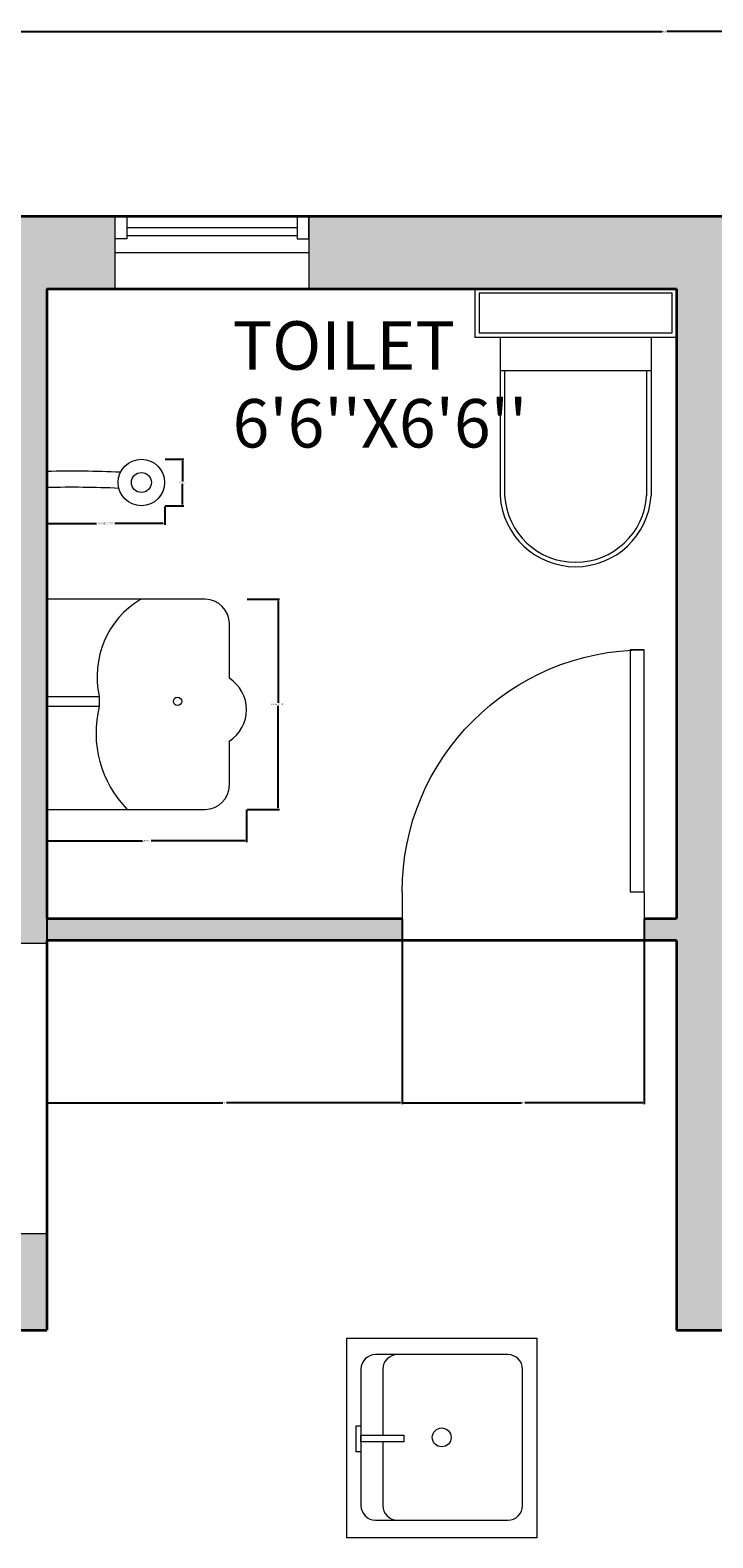
# Model space of a CAD drawing. Units: inches. Extents: x 1789 to 2841, y 3180 to 3702.
# Tile 13 of 14: x 2521 to 2606, y 3491 to 3678. Entities that reach past the tile are written whole.
import ezdxf

# ---------------------------------------------------------------- set-up
doc = ezdxf.new("R2010")
doc.units = ezdxf.units.IN
doc.header["$MEASUREMENT"] = 0
for name, color, linetype, lineweight in [('A-ANNO-DIMS', 2, 'Continuous', 18), ('A-AREA-IDEN', 7, 'Continuous', 18), ('A-FLOR-FIXT', 9, 'Continuous', 18), ('A-WALL', 40, 'Continuous', 35), ('A-WALL-PATT', 252, 'Continuous', 13), ('DORS', 70, 'Continuous', 18), ('WINDOWS', 130, 'Continuous', 18)]:
    doc.layers.add(name, color=color, linetype=linetype, lineweight=lineweight)
doc.styles.get("Standard").update_dxf_attribs({"font": 'arial.ttf'})
doc.dimstyles.get("Standard").update_dxf_attribs({"dimtxt": 0.18, "dimasz": 0.18, "dimexe": 0.18, "dimexo": 0.0625, "dimgap": 0.09, "dimtad": 0, "dimtih": 1, "dimtoh": 1, "dimdec": 0, "dimzin": 0, "dimdsep": 46, "dimlunit": 3, "dimtxsty": 'Standard', "dimcen": 0.09, "dimadec": 0, "dimazin": 0, "dimtfac": 1, "dimtdec": 0, "dimtofl": 0, "dimtmove": 0, "dimatfit": 3, "dimfxl": 1, "dimtolj": 1, "dimtzin": 0, "dimarcsym": 0})

# ---------------------------------------------------------------- blocks, each defined once
blk = doc.blocks.new('HY')
for p, q in [((2053.67, 3653.75), (2074.8, 3653.75)), ((2053.67, 3652.75), (2074.8, 3652.75)), ((2052.23, 3650.66), (2076.23, 3650.66))]:
    blk.add_line(p, q)
for points in [[(2076.23, 3646.16), (2052.23, 3646.16), (2052.23, 3655.16), (2076.23, 3655.16)], [(2052.23, 3655.16), (2053.67, 3655.16), (2053.67, 3652.35), (2052.23, 3652.35)], [(2076.23, 3655.16), (2074.8, 3655.16), (2074.8, 3652.35), (2076.23, 3652.35)]]:
    blk.add_lwpolyline(points, close=True)
blk = doc.blocks.new('GT')
for p, q in [((2141.38, 3640.15), (2141.38, 3620.49)), ((2160.08, 3640.15), (2160.08, 3620.49)), ((2141.38, 3636.04), (2160.08, 3636.04)), ((2141.93, 3636.04), (2141.93, 3620.49)), ((2159.53, 3636.04), (2159.53, 3620.49))]:
    blk.add_line(p, q)
for points in [[(2163.23, 3646.16), (2138.23, 3646.16), (2138.23, 3640.15), (2163.23, 3640.15)], [(2162.68, 3645.61), (2138.78, 3645.61), (2138.78, 3640.7), (2162.68, 3640.7)]]:
    blk.add_lwpolyline(points, close=True)
for radius in [9.37, 8.82]:
    blk.add_arc((2150.73, 3621.09), radius, 183.6546, 356.3454)
blk = doc.blocks.new('*U9')
for p, q in [((0, 0), (0, -6)), ((36, 0), (36, -6))]:
    blk.add_line(p, q)
blk.add_lwpolyline([(0, 0), (0, 36), (1.75, 36), (1.75, 0)], close=True)
blk.add_arc((0, 0), 36, 0, 90)
blk = doc.blocks.new('*U10')
for p, q in [((0, 0), (0, -6)), ((30, 0), (30, -6))]:
    blk.add_line(p, q)
blk.add_lwpolyline([(0, 0), (0, 30), (1.75, 30), (1.75, 0)], close=True)
blk.add_arc((0, 0), 30, 0, 90)
blk = doc.blocks.new('TYTY')
for p, q in [((2104.84, 3607.68), (2085.23, 3607.68)), ((2085.23, 3607.68), (2085.23, 3581.66)), ((2107.84, 3597.9), (2107.84, 3604.68)), ((2107.84, 3584.66), (2107.84, 3590.13)), ((2085.23, 3581.66), (2104.84, 3581.66))]:
    blk.add_line(p, q)
blk.add_lwpolyline([(2085.23, 3595.66), (2091.71, 3595.66), (2091.71, 3594.41), (2085.23, 3594.41)], close=True)
blk.add_circle((2101.42, 3595.04), 0.517)
for centre, radius, start, end in [((2102.58, 3598.14), 11.14, 121.1396, 192.8397), ((2104.84, 3604.68), 3, 0, 90), ((2105.34, 3594.01), 4.62, 302.7804, 57.2196), ((2104.89, 3591.14), 13.58, 166.0641, 224.2681), ((2104.84, 3584.66), 3, 270, 0)]:
    blk.add_arc(centre, radius, start, end)
blk = doc.blocks.new('SINK')
for points in [[(2247.56, 3305.33), (2275.07, 3305.33), (2275.07, 3279.16), (2247.56, 3279.16)], [(2260.91, 3287.01), (2261.87, 3287.01), (2261.87, 3281.09), (2260.91, 3281.09)], [(2259.67, 3281.09), (2263.21, 3281.09), (2263.21, 3280.41), (2259.67, 3280.41)]]:
    blk.add_lwpolyline(points, close=True)
blk.add_lwpolyline([(2251.84, 3281.09), (2270.63, 3281.09, 0.414214), (2272.63, 3283.09), (2272.63, 3301.33, 0.414214), (2270.63, 3303.33), (2251.84, 3303.33, 0.414214), (2249.84, 3301.33), (2249.84, 3283.09, 0.414214)], format="xyb", close=True)
for points in [[(2249.84, 3301.33), (2249.84, 3286.11, 0.414214), (2251.84, 3284.11), (2260.91, 3284.11)], [(2261.87, 3284.11), (2270.63, 3284.11, 0.414214), (2272.63, 3286.11), (2272.63, 3301.33)]]:
    blk.add_lwpolyline(points, format="xyb")
blk.add_circle((2261.24, 3292.21), 1.3)
blk = doc.blocks.new('SOUW')
for radius in [2.88, 1.24]:
    blk.add_circle((2096.93, 3622.15), radius)
for radius, start in [(130.14, 87.3378), (128.14, 87.3891)]:
    blk.add_arc((2088.3, 3493.42), radius, start, 91.3578)
blk = doc.blocks.new('*D51')
at = {"layer": 'A-ANNO-DIMS', "color": 0, "lineweight": -2, "transparency": 16777216}
for p, q in [((2548.02, 3607.68), (2552.04, 3607.68)), ((2551.86, 3607.5), (2551.86, 3594.85)), ((2551.86, 3581.84), (2551.86, 3594.49)), ((2548.02, 3581.66), (2552.04, 3581.66))]:
    blk.add_line(p, q, dxfattribs=at)
at = {"layer": 'A-ANNO-DIMS', "color": 0, "transparency": 16777216}
for points in [[(2551.83, 3607.5), (2551.89, 3607.5), (2551.86, 3607.68)], [(2551.83, 3581.84), (2551.89, 3581.84), (2551.86, 3581.66)]]:
    blk.add_solid(points, dxfattribs=at)
at = {"layer": 'Defpoints', "color": 0, "transparency": 16777216}
for p in [(2547.96, 3607.68), (2551.86, 3607.68), (2547.96, 3581.66)]:
    blk.add_point(p, dxfattribs=at)
at = {"layer": 'A-ANNO-DIMS', "color": 0, "transparency": 16777216, "insert": (2551.86, 3594.67), "char_height": 0.18, "attachment_point": 5}
blk.add_mtext('\\A1;BASIN 26 TYP.', dxfattribs=at)
blk = doc.blocks.new('*D52')
at = {"layer": 'A-ANNO-DIMS', "color": 0, "lineweight": -2, "transparency": 16777216}
for p, q in [((2523.23, 3581.6), (2523.23, 3577.58)), ((2547.96, 3581.6), (2547.96, 3577.58)), ((2523.41, 3577.76), (2535.07, 3577.76)), ((2547.78, 3577.76), (2536.13, 3577.76))]:
    blk.add_line(p, q, dxfattribs=at)
at = {"layer": 'A-ANNO-DIMS', "color": 0, "transparency": 16777216}
for points in [[(2523.41, 3577.79), (2523.41, 3577.73), (2523.23, 3577.76)], [(2547.78, 3577.79), (2547.78, 3577.73), (2547.96, 3577.76)]]:
    blk.add_solid(points, dxfattribs=at)
at = {"layer": 'Defpoints', "color": 0, "transparency": 16777216}
for p in [(2523.23, 3581.66), (2547.96, 3581.66), (2547.96, 3577.76)]:
    blk.add_point(p, dxfattribs=at)
at = {"layer": 'A-ANNO-DIMS', "color": 0, "transparency": 16777216, "insert": (2535.6, 3577.76), "char_height": 0.18, "attachment_point": 5}
blk.add_mtext('\\A1;25 TYP.', dxfattribs=at)
blk = doc.blocks.new('*D57')
at = {"layer": 'A-ANNO-DIMS', "color": 0, "lineweight": -2, "transparency": 16777216}
for p, q in [((2523.22, 3619.2), (2523.22, 3616.9)), ((2537.82, 3619.2), (2537.82, 3616.9)), ((2523.4, 3617.08), (2529.39, 3617.08)), ((2537.64, 3617.08), (2531.65, 3617.08))]:
    blk.add_line(p, q, dxfattribs=at)
at = {"layer": 'A-ANNO-DIMS', "color": 0, "transparency": 16777216}
for points in [[(2523.4, 3617.11), (2523.4, 3617.05), (2523.22, 3617.08)], [(2537.64, 3617.11), (2537.64, 3617.05), (2537.82, 3617.08)]]:
    blk.add_solid(points, dxfattribs=at)
at = {"layer": 'Defpoints', "color": 0, "transparency": 16777216}
for p in [(2523.22, 3619.26), (2537.82, 3619.26), (2537.82, 3617.08)]:
    blk.add_point(p, dxfattribs=at)
at = {"layer": 'A-ANNO-DIMS', "color": 0, "transparency": 16777216, "insert": (2530.52, 3617.08), "char_height": 0.18, "attachment_point": 5}
blk.add_mtext('\\A1;SHOWER 15 TYP.', dxfattribs=at)
blk = doc.blocks.new('*D58')
at = {"layer": 'A-ANNO-DIMS', "color": 0, "lineweight": -2, "transparency": 16777216}
for p, q in [((2537.88, 3625.03), (2540.19, 3625.03)), ((2540.01, 3624.85), (2540.01, 3622.33)), ((2540.01, 3619.44), (2540.01, 3621.97)), ((2537.88, 3619.26), (2540.19, 3619.26))]:
    blk.add_line(p, q, dxfattribs=at)
at = {"layer": 'A-ANNO-DIMS', "color": 0, "transparency": 16777216}
for points in [[(2539.98, 3624.85), (2540.04, 3624.85), (2540.01, 3625.03)], [(2539.98, 3619.44), (2540.04, 3619.44), (2540.01, 3619.26)]]:
    blk.add_solid(points, dxfattribs=at)
at = {"layer": 'Defpoints', "color": 0, "transparency": 16777216}
for p in [(2537.82, 3625.03), (2540.01, 3625.03), (2537.82, 3619.26)]:
    blk.add_point(p, dxfattribs=at)
at = {"layer": 'A-ANNO-DIMS', "color": 0, "transparency": 16777216, "insert": (2540.01, 3622.15), "char_height": 0.18, "attachment_point": 5}
blk.add_mtext('\\A1;6 TYP.', dxfattribs=at)
blk = doc.blocks.new('*D95')
at = {"layer": 'A-ANNO-DIMS', "color": 0, "lineweight": -2, "transparency": 16777216}
for p, q in [((2397.23, 3655.22), (2397.23, 3678.19)), ((2397.41, 3678.01), (2599.44, 3678.01)), ((2802.05, 3678.01), (2600.03, 3678.01)), ((2802.23, 3526.22), (2802.23, 3678.19))]:
    blk.add_line(p, q, dxfattribs=at)
at = {"layer": 'A-ANNO-DIMS', "color": 0, "transparency": 16777216}
for points in [[(2397.41, 3678.04), (2397.41, 3677.98), (2397.23, 3678.01)], [(2802.05, 3678.04), (2802.05, 3677.98), (2802.23, 3678.01)]]:
    blk.add_solid(points, dxfattribs=at)
at = {"layer": 'Defpoints', "color": 0, "transparency": 16777216}
for p in [(2802.23, 3678.01), (2397.23, 3655.16), (2802.23, 3526.16)]:
    blk.add_point(p, dxfattribs=at)
at = {"layer": 'A-ANNO-DIMS', "color": 0, "transparency": 16777216, "insert": (2599.73, 3678.01), "char_height": 0.18, "attachment_point": 5}
blk.add_mtext('\\A1;405', dxfattribs=at)
blk = doc.blocks.new('*D107')
at = {"layer": 'A-ANNO-DIMS', "color": 0, "lineweight": -2, "transparency": 16777216}
for p, q in [((2523.23, 3568.1), (2523.23, 3545.13)), ((2567.23, 3568.1), (2567.23, 3545.13)), ((2523.41, 3545.31), (2545.01, 3545.31)), ((2567.05, 3545.31), (2545.46, 3545.31))]:
    blk.add_line(p, q, dxfattribs=at)
at = {"layer": 'A-ANNO-DIMS', "color": 0, "transparency": 16777216}
for points in [[(2523.41, 3545.34), (2523.41, 3545.28), (2523.23, 3545.31)], [(2567.05, 3545.34), (2567.05, 3545.28), (2567.23, 3545.31)]]:
    blk.add_solid(points, dxfattribs=at)
at = {"layer": 'Defpoints', "color": 0, "transparency": 16777216}
for p in [(2523.23, 3568.16), (2567.23, 3568.16), (2523.23, 3545.31)]:
    blk.add_point(p, dxfattribs=at)
at = {"layer": 'A-ANNO-DIMS', "color": 0, "transparency": 16777216, "insert": (2545.23, 3545.31), "char_height": 0.18, "attachment_point": 5}
blk.add_mtext('\\A1;44', dxfattribs=at)
blk = doc.blocks.new('*D108')
at = {"layer": 'A-ANNO-DIMS', "color": 0, "lineweight": -2, "transparency": 16777216}
for p, q in [((2567.23, 3568.1), (2567.23, 3545.13)), ((2597.23, 3568.1), (2597.23, 3545.13)), ((2567.41, 3545.31), (2582.01, 3545.31)), ((2597.05, 3545.31), (2582.45, 3545.31))]:
    blk.add_line(p, q, dxfattribs=at)
at = {"layer": 'A-ANNO-DIMS', "color": 0, "transparency": 16777216}
for points in [[(2567.41, 3545.34), (2567.41, 3545.28), (2567.23, 3545.31)], [(2597.05, 3545.34), (2597.05, 3545.28), (2597.23, 3545.31)]]:
    blk.add_solid(points, dxfattribs=at)
at = {"layer": 'Defpoints', "color": 0, "transparency": 16777216}
for p in [(2567.23, 3568.16), (2597.23, 3568.16), (2567.23, 3545.31)]:
    blk.add_point(p, dxfattribs=at)
at = {"layer": 'A-ANNO-DIMS', "color": 0, "transparency": 16777216, "insert": (2582.23, 3545.31), "char_height": 0.18, "attachment_point": 5}
blk.add_mtext('\\A1;30', dxfattribs=at)

msp = doc.modelspace()

# ---------------------------------------------------------------- hatches: boundary and pattern name
at = {"layer": 'A-WALL-PATT'}
h = msp.add_hatch(color=256, dxfattribs=at)
h.dxf.hatch_style = 1
h.paths.add_polyline_path([(2490.2333, 3655.1608), (2397.2333, 3655.1608), (2397.2333, 3622.3936), (2406.2333, 3622.3936), (2406.2333, 3646.1608), (2490.2333, 3646.1608)])
h.paths.add_polyline_path([(2642.4325, 3655.1608), (2555.6786, 3655.1608), (2555.6786, 3646.1608), (2601.2333, 3646.1608), (2601.2333, 3640.1475), (2601.2333, 3568.1608), (2597.2333, 3568.1608), (2597.2333, 3565.4274), (2601.2333, 3565.4274), (2601.2333, 3528.1608), (2601.2333, 3517.1608), (2612.9879, 3517.1608), (2613.0522, 3523.352), (2613.0813, 3526.1608), (2610.2333, 3526.1608), (2610.2333, 3646.1608), (2634.2333, 3646.1608), (2642.4325, 3646.1608)])
h.paths.add_polyline_path([(2523.2333, 3646.1608), (2531.6786, 3646.1608), (2531.6786, 3655.1608), (2514.2333, 3655.1608), (2514.2333, 3646.1608), (2514.2333, 3621.0865), (2514.2333, 3564.976, -0.02086055), (2517.2333, 3565.1012), (2523.2333, 3565.1012), (2523.2333, 3565.4274), (2567.2333, 3565.4274), (2567.2333, 3568.1608), (2523.2333, 3568.1608)])
h = msp.add_hatch(color=256, dxfattribs=at)
h.dxf.hatch_style = 1
h.paths.add_polyline_path([(2406.2333, 3517.1608), (2461.6918, 3517.1608), (2461.6918, 3517.6724), (2477.6863, 3517.6724), (2523.2333, 3517.1608), (2523.2333, 3529.1012), (2516.8782, 3529.1012), (2516.8782, 3526.1608), (2406.2333, 3526.1608), (2406.2333, 3562.3936), (2397.2333, 3562.3936), (2397.2333, 3513.1608), (2403.2333, 3513.1608), (2406.2333, 3513.1608)])

# ---------------------------------------------------------------- linework, layer by layer
at = {"layer": 'A-WALL'}
for p, q in [((2397.2333, 3655.1608), (2763.2333, 3655.1608)), ((2523.2333, 3646.1608), (2523.2333, 3568.1608)), ((2523.2333, 3646.1608), (2601.2333, 3646.1608)), ((2601.2333, 3646.1608), (2601.2333, 3568.1608)), ((2523.2333, 3568.1608), (2567.2333, 3568.1608)), ((2597.2333, 3568.1608), (2601.2333, 3568.1608)), ((2523.2333, 3565.4274), (2523.2333, 3517.1608)), ((2601.2333, 3565.4274), (2523.2333, 3565.4274)), ((2601.2333, 3565.4274), (2601.2333, 3528.1608)), ((2601.2333, 3528.1608), (2601.2333, 3517.1608)), ((2406.2333, 3517.1608), (2523.2333, 3517.1608)), ((2601.2333, 3517.1608), (2721.2333, 3517.1608))]:
    msp.add_line(p, q, dxfattribs=at)

# ---------------------------------------------------------------- block references
at = {"layer": 'A-FLOR-FIXT'}
for name in ['GT', 'SOUW', 'TYTY']:
    msp.add_blockref(name, (438, 0), dxfattribs=at)
at = {"layer": 'A-FLOR-FIXT', "xscale": 0.8998033160254596, "yscale": 0.8998033160254596, "zscale": 0.8998033160254596, "rotation": 270}
msp.add_blockref('SINK', (-390.2004, 5538.5297), dxfattribs=at)
at = {"layer": 'DORS', "xscale": -1}
msp.add_blockref('*U10', (2597.2333, 3571.4274), dxfattribs=at)
at = {"layer": 'DORS', "rotation": 90.00000000000003}
msp.add_blockref('*U9', (2517.2333, 3529.1012), dxfattribs=at)
at = {"layer": 'WINDOWS'}
msp.add_blockref('HY', (479.4453, 0), dxfattribs=at)

# ---------------------------------------------------------------- texts
at = {"layer": 'A-ANNO-DIMS'}
msp.add_text("6'6''X6'6''", height=6, dxfattribs=at).set_placement((2546.2402, 3626.4874))
at = {"layer": 'A-AREA-IDEN'}
msp.add_text('TOILET', height=6, dxfattribs=at).set_placement((2546.2402, 3636.1259))

# ---------------------------------------------------------------- dimensions: what is measured, and where the dimension line sits
at = {"layer": 'A-ANNO-DIMS'}
dim = msp.add_linear_dim(base=(2802.2333, 3678.0108), p1=(2397.2333, 3655.1608), p2=(2802.2333, 3526.1608), dimstyle='Standard', override={"dimdec": 0, "dimlfac": 1, "dimrnd": 0, "dimzin": 0, "dimdsep": 46, "dimlunit": 2}, dxfattribs=at)
dim.commit()
dim.dimension.update_dxf_attribs({"geometry": '*D95', "text_midpoint": (2599.7333, 3678.0108)})
for base, p1, p2, text, picture, middle in [((2540.005, 3625.03), (2537.8157, 3619.2649), (2537.8157, 3625.03), '<> TYP.', '*D58', (2540.005, 3622.1474)), ((2551.865, 3607.6776), (2547.9625, 3581.6608), (2547.9625, 3607.6776), 'BASIN <> TYP.', '*D51', (2551.865, 3594.6692))]:
    dim = msp.add_linear_dim(base=base, p1=p1, p2=p2, angle=90, text=text, dimstyle='Standard', override={"dimdec": 0, "dimlfac": 1, "dimrnd": 0, "dimzin": 0, "dimdsep": 46, "dimlunit": 2}, dxfattribs=at)
    dim.commit()
    dim.dimension.update_dxf_attribs({"geometry": picture, "text_midpoint": middle})
for base, p1, p2, text, picture, middle in [((2537.8157, 3617.0756), (2523.2199, 3619.2649), (2537.8157, 3619.2649), 'SHOWER <> TYP.', '*D57', (2530.5178, 3617.0756)), ((2547.9625, 3577.7583), (2523.2333, 3581.6608), (2547.9625, 3581.6608), '<> TYP.', '*D52', (2535.5979, 3577.7583))]:
    dim = msp.add_linear_dim(base=base, p1=p1, p2=p2, text=text, dimstyle='Standard', override={"dimdec": 0, "dimlfac": 1, "dimrnd": 0, "dimzin": 0, "dimdsep": 46, "dimlunit": 2}, dxfattribs=at)
    dim.commit()
    dim.dimension.update_dxf_attribs({"geometry": picture, "text_midpoint": middle})
for base, p1, p2, picture, middle in [((2523.2333, 3545.3108), (2567.2333, 3568.1608), (2523.2333, 3568.1608), '*D107', (2545.2333, 3545.3108)), ((2567.2333, 3545.3108), (2597.2333, 3568.1608), (2567.2333, 3568.1608), '*D108', (2582.2333, 3545.3108))]:
    dim = msp.add_linear_dim(base=base, p1=p1, p2=p2, angle=180, dimstyle='Standard', override={"dimdec": 0, "dimlfac": 1, "dimrnd": 0, "dimzin": 0, "dimdsep": 46, "dimlunit": 2}, dxfattribs=at)
    dim.commit()
    dim.dimension.update_dxf_attribs({"geometry": picture, "text_midpoint": middle})

doc.saveas('drawing.dxf')
